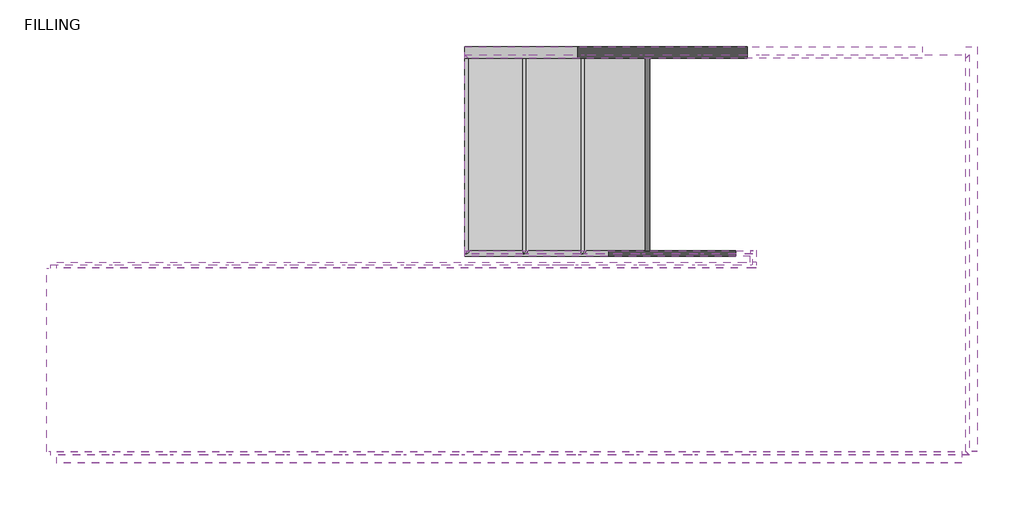
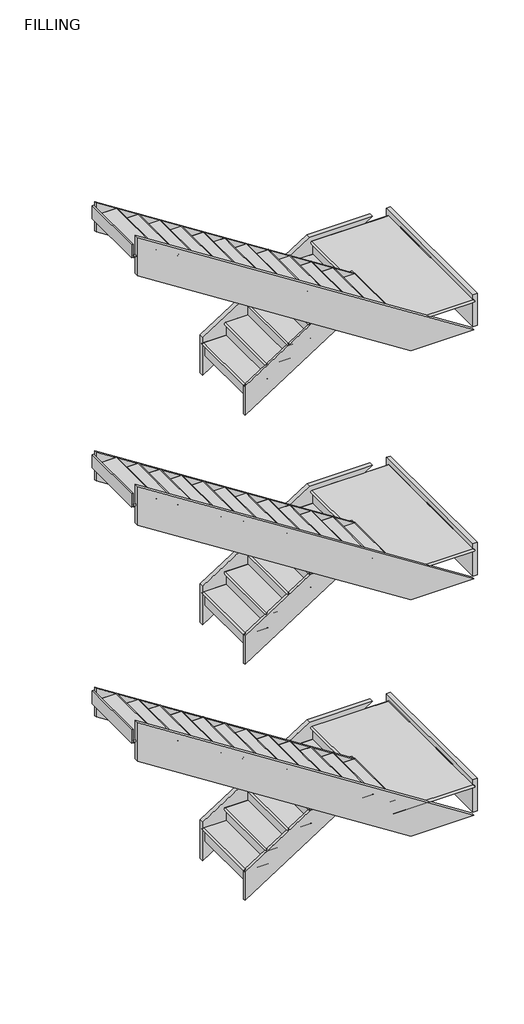
# One storey, incomplete: 18 members, 3 stair flights.
"""IFC4 building model written with IfcOpenShell, lengths in millimetres."""

from ifc_helpers import new_model, si_unit, frame, origin, place, context, project, spatial, polyline, outline, extrude, transform, mapped, element, save
from components import wood_steps_w_30mm_tread_25mm_nosing_19mm_riser_5243a390, wood_steps_w_30mm_tread_25mm_nosing_19mm_riser_1d491615, wood_steps_w_30mm_tread_25mm_nosing_19mm_riser_de9e5e1f

model = new_model("IFC4")

# Units and contexts
model_context = context("Model", 3, world=origin())
ifc_project = project(units=[si_unit("LENGTHUNIT", "METRE", prefix="MILLI")], contexts=[model_context])

# Site, building, storey
site = spatial("IfcSite", under=ifc_project)
building = spatial("IfcBuilding", under=site)
storey = spatial("IfcBuildingStorey", under=building, Name="FILLING", Elevation=0.0)

# Members
placement = place(None, origin())
element("IfcMember", 1, at=placement, inside=storey, context=model_context, shape_type="SweptSolid", body=[
    extrude(outline(polyline([(3812.5003181, -8680.149573), (3337.6244209, -8680.149573), (4614.1165081, -6685.1910414), (4614.1165081, -7427.348186), (3812.5003181, -8680.149573)])), frame((0.0, -10219.6521308, 0.0), z_axis=(0.0, 1.0, 0.0), x_axis=(0.0, 0.0, 1.0)), (0.0, 0.0, 1.0), 50.0),
])
element("IfcMember", 2, at=placement, inside=storey, context=model_context, shape_type="SweptSolid", body=[
    extrude(outline(polyline([(-6495.4132565, -10169.6521308), (-6445.4132565, -10169.6521308), (-6445.4132565, -11934.0860066), (-6495.4132565, -11934.0860066), (-6495.4132565, -10169.6521308)])), frame((0.0, 0.0, 4214.1165081), z_axis=(0.0, 0.0, 1.0), x_axis=(1.0, 0.0, 0.0)), (0.0, 0.0, 1.0), 400.0),
])
element("IfcMember", 3, at=placement, inside=storey, context=model_context, shape_type="SweptSolid", body=[
    extrude(outline(polyline([(4214.1165081, -6513.1111248), (6738.8105082, -10457.8773536), (6263.9018177, -10457.8773536), (4214.1165081, -7255.143135), (4214.1165081, -6513.1111248)])), frame((0.0, -11984.0860066, 0.0), z_axis=(0.0, 1.0, 0.0), x_axis=(0.0, 0.0, 1.0)), (0.0, 0.0, 1.0), 50.0),
])
element("IfcMember", 4, at=placement, inside=storey, context=model_context, shape_type="SweptSolid", body=[
    extrude(outline(polyline([(3725.8354669, -8680.149573), (3369.678544, -8680.149573), (4166.571014, -7434.7306254), (4522.7279369, -7434.7306254), (3725.8354669, -8680.149573)])), frame((0.0, -11083.3255223, 0.0), z_axis=(0.0, 1.0, 0.0), x_axis=(0.0, 0.0, 1.0)), (0.0, 0.0, 1.0), 25.0),
])
element("IfcMember", 5, at=placement, inside=storey, context=model_context, shape_type="SweptSolid", body=[
    extrude(outline(polyline([(-7434.7306254, -11058.3255223), (-7409.7306254, -11058.3255223), (-7409.7306254, -11109.5255223), (-7434.7306254, -11109.5255223), (-7434.7306254, -11058.3255223)])), frame((0.0, 0.0, 4396.68), z_axis=(0.0, 0.0, 1.0), x_axis=(1.0, 0.0, 0.0)), (0.0, 0.0, 1.0), 300.0),
])
element("IfcMember", 6, at=placement, inside=storey, context=model_context, shape_type="SweptSolid", body=[
    extrude(outline(polyline([(4396.68, -7409.7306254), (4701.2920656, -7409.7306254), (6652.1396722, -10457.8773536), (6295.9581543, -10457.8773536), (4396.68, -7490.3065026), (4396.68, -7409.7306254)])), frame((0.0, -11134.5255223, 0.0), z_axis=(0.0, 1.0, 0.0), x_axis=(0.0, 0.0, 1.0)), (0.0, 0.0, 1.0), 25.0),
])
element("IfcMember", 7, at=placement, inside=storey, context=model_context, shape_type="SweptSolid", body=[
    extrude(outline(polyline([(6901.1403181, -8680.149573), (6426.2644209, -8680.149573), (7702.7565081, -6685.1910414), (7702.7565081, -7427.348186), (6901.1403181, -8680.149573)])), frame((0.0, -10219.6521308, 0.0), z_axis=(0.0, 1.0, 0.0), x_axis=(0.0, 0.0, 1.0)), (0.0, 0.0, 1.0), 50.0),
])
element("IfcMember", 8, at=placement, inside=storey, context=model_context, shape_type="SweptSolid", body=[
    extrude(outline(polyline([(-6495.4132565, -10169.6521308), (-6445.4132565, -10169.6521308), (-6445.4132565, -11934.0860066), (-6495.4132565, -11934.0860066), (-6495.4132565, -10169.6521308)])), frame((0.0, 0.0, 7302.7565081), z_axis=(0.0, 0.0, 1.0), x_axis=(1.0, 0.0, 0.0)), (0.0, 0.0, 1.0), 400.0),
])
element("IfcMember", 9, at=placement, inside=storey, context=model_context, shape_type="SweptSolid", body=[
    extrude(outline(polyline([(7302.7565081, -6513.1111248), (9827.4505082, -10457.8773536), (9352.5418177, -10457.8773536), (7302.7565081, -7255.143135), (7302.7565081, -6513.1111248)])), frame((0.0, -11984.0860066, 0.0), z_axis=(0.0, 1.0, 0.0), x_axis=(0.0, 0.0, 1.0)), (0.0, 0.0, 1.0), 50.0),
])
element("IfcMember", 10, at=placement, inside=storey, context=model_context, shape_type="SweptSolid", body=[
    extrude(outline(polyline([(6814.4754669, -8680.149573), (6458.318544, -8680.149573), (7255.211014, -7434.7306254), (7611.3679369, -7434.7306254), (6814.4754669, -8680.149573)])), frame((0.0, -11083.3255223, 0.0), z_axis=(0.0, 1.0, 0.0), x_axis=(0.0, 0.0, 1.0)), (0.0, 0.0, 1.0), 25.0),
])
element("IfcMember", 11, at=placement, inside=storey, context=model_context, shape_type="SweptSolid", body=[
    extrude(outline(polyline([(-7434.7306254, -11058.3255223), (-7409.7306254, -11058.3255223), (-7409.7306254, -11109.5255223), (-7434.7306254, -11109.5255223), (-7434.7306254, -11058.3255223)])), frame((0.0, 0.0, 7485.32), z_axis=(0.0, 0.0, 1.0), x_axis=(1.0, 0.0, 0.0)), (0.0, 0.0, 1.0), 300.0),
])
element("IfcMember", 12, at=placement, inside=storey, context=model_context, shape_type="SweptSolid", body=[
    extrude(outline(polyline([(7485.32, -7409.7306254), (7789.9320656, -7409.7306254), (9740.7796722, -10457.8773536), (9384.5981543, -10457.8773536), (7485.32, -7490.3065026), (7485.32, -7409.7306254)])), frame((0.0, -11134.5255223, 0.0), z_axis=(0.0, 1.0, 0.0), x_axis=(0.0, 0.0, 1.0)), (0.0, 0.0, 1.0), 25.0),
])
element("IfcMember", 13, ObjectType="Stringer-50mm_Width", at=placement, inside=storey, context=model_context, shape_type="SweptSolid", body=[
    extrude(outline(polyline([(886.4203181, -8680.149573), (411.5444209, -8680.149573), (1688.0365081, -6685.1910414), (1688.0365081, -7427.348186), (886.4203181, -8680.149573)])), frame((0.0, -10219.6521308, 0.0), z_axis=(0.0, 1.0, 0.0), x_axis=(0.0, 0.0, 1.0)), (0.0, 0.0, 1.0), 50.0),
])
element("IfcMember", 14, ObjectType="Stringer-50mm_Width", at=placement, inside=storey, context=model_context, shape_type="SweptSolid", body=[
    extrude(outline(polyline([(-6495.4132565, -10169.6521308), (-6445.4132565, -10169.6521308), (-6445.4132565, -11934.0860066), (-6495.4132565, -11934.0860066), (-6495.4132565, -10169.6521308)])), frame((0.0, 0.0, 1288.0365081), z_axis=(0.0, 0.0, 1.0), x_axis=(1.0, 0.0, 0.0)), (0.0, 0.0, 1.0), 400.0),
])
element("IfcMember", 15, ObjectType="Stringer-50mm_Width", at=placement, inside=storey, context=model_context, shape_type="SweptSolid", body=[
    extrude(outline(polyline([(1288.0365081, -6513.1111248), (3812.7305082, -10457.8773536), (3337.8218177, -10457.8773536), (1288.0365081, -7255.143135), (1288.0365081, -6513.1111248)])), frame((0.0, -11984.0860066, 0.0), z_axis=(0.0, 1.0, 0.0), x_axis=(0.0, 0.0, 1.0)), (0.0, 0.0, 1.0), 50.0),
])
element("IfcMember", 16, ObjectType="Stringer-50mm_Width", at=placement, inside=storey, context=model_context, shape_type="SweptSolid", body=[
    extrude(outline(polyline([(799.7554669, -8680.149573), (443.598544, -8680.149573), (1240.491014, -7434.7306254), (1596.6479369, -7434.7306254), (799.7554669, -8680.149573)])), frame((0.0, -11083.3255223, 0.0), z_axis=(0.0, 1.0, 0.0), x_axis=(0.0, 0.0, 1.0)), (0.0, 0.0, 1.0), 25.0),
])
element("IfcMember", 17, ObjectType="Stringer-50mm_Width", at=placement, inside=storey, context=model_context, shape_type="SweptSolid", body=[
    extrude(outline(polyline([(-7434.7306254, -11058.3255223), (-7409.7306254, -11058.3255223), (-7409.7306254, -11109.5255223), (-7434.7306254, -11109.5255223), (-7434.7306254, -11058.3255223)])), frame((0.0, 0.0, 1470.6), z_axis=(0.0, 0.0, 1.0), x_axis=(1.0, 0.0, 0.0)), (0.0, 0.0, 1.0), 300.0),
])
element("IfcMember", 18, ObjectType="Stringer-50mm_Width", at=placement, inside=storey, context=model_context, shape_type="SweptSolid", body=[
    extrude(outline(polyline([(1470.6, -7409.7306254), (1775.2120656, -7409.7306254), (3726.0596722, -10457.8773536), (3369.8781543, -10457.8773536), (1470.6, -7490.3065026), (1470.6, -7409.7306254)])), frame((0.0, -11134.5255223, 0.0), z_axis=(0.0, 1.0, 0.0), x_axis=(0.0, 0.0, 1.0)), (0.0, 0.0, 1.0), 25.0),
])

# Stair flights
wood_steps_w_30mm_tread_25mm_nosing_19mm_riser_shape = wood_steps_w_30mm_tread_25mm_nosing_19mm_riser_5243a390(model_context)
element("IfcStairFlight", 19, ObjectType="Wood_Steps_w-30mm_Tread-25mm_Nosing-19mm_Riser", at=placement, inside=storey, context=model_context, shape_type="MappedRepresentation", body=[
    mapped(wood_steps_w_30mm_tread_25mm_nosing_19mm_riser_shape, transform((0.0, 0.0, 0.0), x_axis=(1.0, 0.0, 0.0), y_axis=(0.0, 1.0, 0.0), z_axis=(0.0, 0.0, 1.0))),
])
wood_steps_w_30mm_tread_25mm_nosing_19mm_riser_2_shape = wood_steps_w_30mm_tread_25mm_nosing_19mm_riser_1d491615(model_context)
element("IfcStairFlight", 20, ObjectType="Wood_Steps_w-30mm_Tread-25mm_Nosing-19mm_Riser", at=placement, inside=storey, context=model_context, shape_type="MappedRepresentation", body=[
    mapped(wood_steps_w_30mm_tread_25mm_nosing_19mm_riser_2_shape, transform((0.0, 0.0, 0.0), x_axis=(1.0, 0.0, 0.0), y_axis=(0.0, 1.0, 0.0), z_axis=(0.0, 0.0, 1.0))),
])
wood_steps_w_30mm_tread_25mm_nosing_19mm_riser_3_shape = wood_steps_w_30mm_tread_25mm_nosing_19mm_riser_de9e5e1f(model_context)
element("IfcStairFlight", 21, ObjectType="Wood_Steps_w-30mm_Tread-25mm_Nosing-19mm_Riser", at=placement, inside=storey, context=model_context, shape_type="MappedRepresentation", body=[
    mapped(wood_steps_w_30mm_tread_25mm_nosing_19mm_riser_3_shape, transform((0.0, 0.0, 0.0), x_axis=(1.0, 0.0, 0.0), y_axis=(0.0, 1.0, 0.0), z_axis=(0.0, 0.0, 1.0))),
])

save(model, "model.ifc")

# Revit data of these elements
# Elements 1, 2, 3, 7, 8, 9 (IfcMember)
#   Phase Created = New Construction
# Elements 4, 5, 6, 10, 11, 12 (IfcMember)
#   Phase Created = New Construction
#   Materials on its faces: "Wood"
# Elements 13, 14, 15 (IfcMember, "Stringer-50mm_Width")
#   Phase Created = New Construction
# Elements 16, 17, 18 (IfcMember, "Stringer-50mm_Width")
#   Phase Created = New Construction
#   Materials on its faces: "Wood"
# Elements 19, 20, 21 (IfcStairFlight, "Wood_Steps_w-30mm_Tread-25mm_Nosing-19mm_Riser")
#   Phase Created = New Construction
#   Materials on its faces: "Wood", "Cherry"
# Materials
#   "Wood": class "Wood", colour RGB 212 179 113, transparency 0, Description = "Generic wood", Cost = 0
#   "Cherry": class "Wood", colour RGB 226 177 128, transparency 0, Description = "Prunus Serotina", Cost = 0
